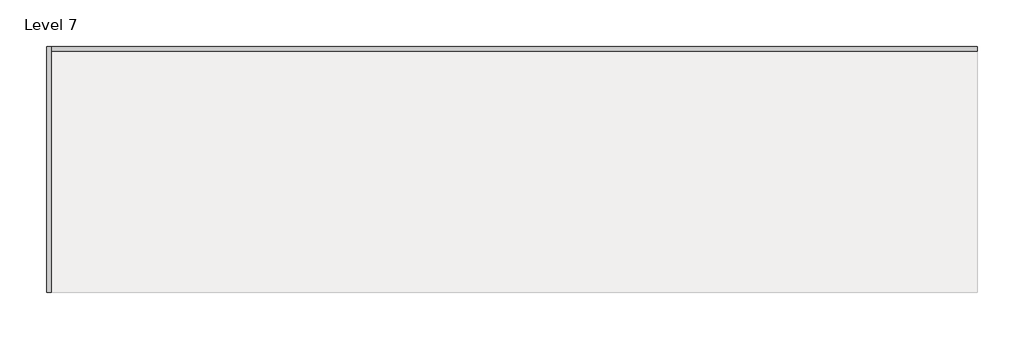
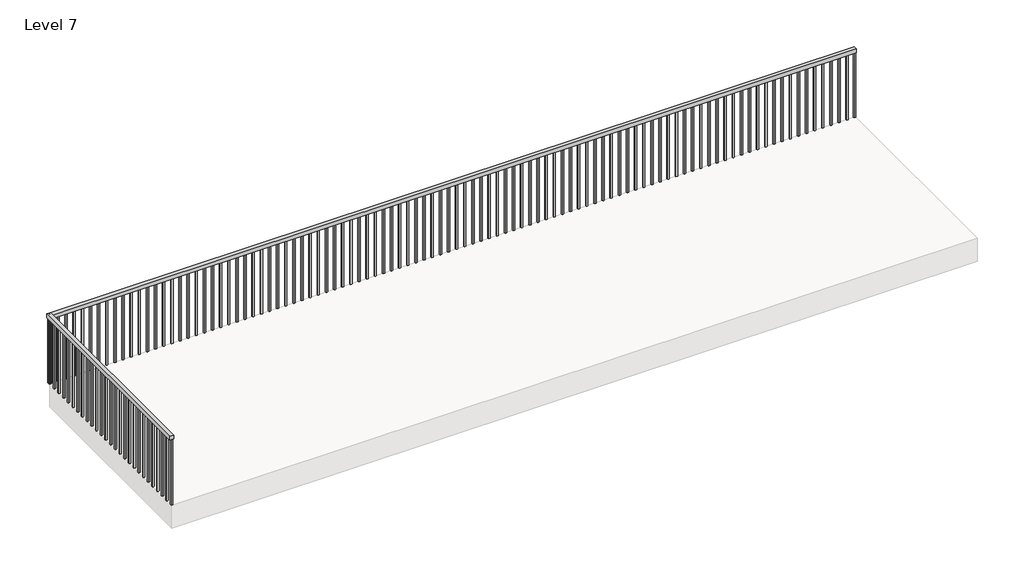
# One storey, part 3 of 5: 2 railings.
"""IFC4 building model written with IfcOpenShell, lengths in millimetres."""

from ifc_helpers import new_model, si_unit, frame, origin, place, context, project, spatial, polyline, outline, extrude, element, save

model = new_model("IFC4")

# Units and contexts
model_context = context("Model", 3, world=origin())
ifc_project = project(units=[si_unit("LENGTHUNIT", "METRE", prefix="MILLI")], contexts=[model_context])

# Site, building, storey
site = spatial("IfcSite", under=ifc_project)
building = spatial("IfcBuilding", under=site)
storey = spatial("IfcBuildingStorey", under=building, Name="Level 7", Elevation=6400.8)

# Railings
placement = place(None, origin())
element("IfcRailing", 1, ObjectType="Handrail - Rectangular", at=placement, inside=storey, context=model_context, shape_type="SweptSolid", body=[
    extrude(outline(polyline([(-13833.4638778, 17384.8237525), (-13833.4638778, 17435.6237525), (-3775.0638778, 17435.6237525), (-3775.0638778, 17384.8237525), (-13833.4638778, 17384.8237525)])), frame((0.0, 0.0, 7264.4), z_axis=(0.0, 0.0, 1.0), x_axis=(1.0, 0.0, 0.0)), (0.0, 0.0, 1.0), 50.8),
    extrude(outline(polyline([(-3886.1888778, 17400.6987525), (-3886.1888778, 17419.7487525), (-3867.1388778, 17419.7487525), (-3867.1388778, 17400.6987525), (-3886.1888778, 17400.6987525)])), frame((0.0, 0.0, 6400.8), z_axis=(0.0, 0.0, 1.0), x_axis=(1.0, 0.0, 0.0)), (0.0, 0.0, 1.0), 863.6),
    extrude(outline(polyline([(-3987.7888778, 17400.6987525), (-3987.7888778, 17419.7487525), (-3968.7388778, 17419.7487525), (-3968.7388778, 17400.6987525), (-3987.7888778, 17400.6987525)])), frame((0.0, 0.0, 6400.8), z_axis=(0.0, 0.0, 1.0), x_axis=(1.0, 0.0, 0.0)), (0.0, 0.0, 1.0), 863.6),
    extrude(outline(polyline([(-4089.3888778, 17400.6987525), (-4089.3888778, 17419.7487525), (-4070.3388778, 17419.7487525), (-4070.3388778, 17400.6987525), (-4089.3888778, 17400.6987525)])), frame((0.0, 0.0, 6400.8), z_axis=(0.0, 0.0, 1.0), x_axis=(1.0, 0.0, 0.0)), (0.0, 0.0, 1.0), 863.6),
    extrude(outline(polyline([(-4190.9888778, 17400.6987525), (-4190.9888778, 17419.7487525), (-4171.9388778, 17419.7487525), (-4171.9388778, 17400.6987525), (-4190.9888778, 17400.6987525)])), frame((0.0, 0.0, 6400.8), z_axis=(0.0, 0.0, 1.0), x_axis=(1.0, 0.0, 0.0)), (0.0, 0.0, 1.0), 863.6),
    extrude(outline(polyline([(-4292.5888778, 17400.6987525), (-4292.5888778, 17419.7487525), (-4273.5388778, 17419.7487525), (-4273.5388778, 17400.6987525), (-4292.5888778, 17400.6987525)])), frame((0.0, 0.0, 6400.8), z_axis=(0.0, 0.0, 1.0), x_axis=(1.0, 0.0, 0.0)), (0.0, 0.0, 1.0), 863.6),
    extrude(outline(polyline([(-4394.1888778, 17400.6987525), (-4394.1888778, 17419.7487525), (-4375.1388778, 17419.7487525), (-4375.1388778, 17400.6987525), (-4394.1888778, 17400.6987525)])), frame((0.0, 0.0, 6400.8), z_axis=(0.0, 0.0, 1.0), x_axis=(1.0, 0.0, 0.0)), (0.0, 0.0, 1.0), 863.6),
    extrude(outline(polyline([(-4495.7888778, 17400.6987525), (-4495.7888778, 17419.7487525), (-4476.7388778, 17419.7487525), (-4476.7388778, 17400.6987525), (-4495.7888778, 17400.6987525)])), frame((0.0, 0.0, 6400.8), z_axis=(0.0, 0.0, 1.0), x_axis=(1.0, 0.0, 0.0)), (0.0, 0.0, 1.0), 863.6),
    extrude(outline(polyline([(-4597.3888778, 17400.6987525), (-4597.3888778, 17419.7487525), (-4578.3388778, 17419.7487525), (-4578.3388778, 17400.6987525), (-4597.3888778, 17400.6987525)])), frame((0.0, 0.0, 6400.8), z_axis=(0.0, 0.0, 1.0), x_axis=(1.0, 0.0, 0.0)), (0.0, 0.0, 1.0), 863.6),
    extrude(outline(polyline([(-4698.9888778, 17400.6987525), (-4698.9888778, 17419.7487525), (-4679.9388778, 17419.7487525), (-4679.9388778, 17400.6987525), (-4698.9888778, 17400.6987525)])), frame((0.0, 0.0, 6400.8), z_axis=(0.0, 0.0, 1.0), x_axis=(1.0, 0.0, 0.0)), (0.0, 0.0, 1.0), 863.6),
    extrude(outline(polyline([(-4800.5888778, 17400.6987525), (-4800.5888778, 17419.7487525), (-4781.5388778, 17419.7487525), (-4781.5388778, 17400.6987525), (-4800.5888778, 17400.6987525)])), frame((0.0, 0.0, 6400.8), z_axis=(0.0, 0.0, 1.0), x_axis=(1.0, 0.0, 0.0)), (0.0, 0.0, 1.0), 863.6),
    extrude(outline(polyline([(-4902.1888778, 17400.6987525), (-4902.1888778, 17419.7487525), (-4883.1388778, 17419.7487525), (-4883.1388778, 17400.6987525), (-4902.1888778, 17400.6987525)])), frame((0.0, 0.0, 6400.8), z_axis=(0.0, 0.0, 1.0), x_axis=(1.0, 0.0, 0.0)), (0.0, 0.0, 1.0), 863.6),
    extrude(outline(polyline([(-5003.7888778, 17400.6987525), (-5003.7888778, 17419.7487525), (-4984.7388778, 17419.7487525), (-4984.7388778, 17400.6987525), (-5003.7888778, 17400.6987525)])), frame((0.0, 0.0, 6400.8), z_axis=(0.0, 0.0, 1.0), x_axis=(1.0, 0.0, 0.0)), (0.0, 0.0, 1.0), 863.6),
    extrude(outline(polyline([(-5105.3888778, 17400.6987525), (-5105.3888778, 17419.7487525), (-5086.3388778, 17419.7487525), (-5086.3388778, 17400.6987525), (-5105.3888778, 17400.6987525)])), frame((0.0, 0.0, 6400.8), z_axis=(0.0, 0.0, 1.0), x_axis=(1.0, 0.0, 0.0)), (0.0, 0.0, 1.0), 863.6),
    extrude(outline(polyline([(-5206.9888778, 17400.6987525), (-5206.9888778, 17419.7487525), (-5187.9388778, 17419.7487525), (-5187.9388778, 17400.6987525), (-5206.9888778, 17400.6987525)])), frame((0.0, 0.0, 6400.8), z_axis=(0.0, 0.0, 1.0), x_axis=(1.0, 0.0, 0.0)), (0.0, 0.0, 1.0), 863.6),
    extrude(outline(polyline([(-5308.5888778, 17400.6987525), (-5308.5888778, 17419.7487525), (-5289.5388778, 17419.7487525), (-5289.5388778, 17400.6987525), (-5308.5888778, 17400.6987525)])), frame((0.0, 0.0, 6400.8), z_axis=(0.0, 0.0, 1.0), x_axis=(1.0, 0.0, 0.0)), (0.0, 0.0, 1.0), 863.6),
    extrude(outline(polyline([(-5410.1888778, 17400.6987525), (-5410.1888778, 17419.7487525), (-5391.1388778, 17419.7487525), (-5391.1388778, 17400.6987525), (-5410.1888778, 17400.6987525)])), frame((0.0, 0.0, 6400.8), z_axis=(0.0, 0.0, 1.0), x_axis=(1.0, 0.0, 0.0)), (0.0, 0.0, 1.0), 863.6),
    extrude(outline(polyline([(-5511.7888778, 17400.6987525), (-5511.7888778, 17419.7487525), (-5492.7388778, 17419.7487525), (-5492.7388778, 17400.6987525), (-5511.7888778, 17400.6987525)])), frame((0.0, 0.0, 6400.8), z_axis=(0.0, 0.0, 1.0), x_axis=(1.0, 0.0, 0.0)), (0.0, 0.0, 1.0), 863.6),
    extrude(outline(polyline([(-5613.3888778, 17400.6987525), (-5613.3888778, 17419.7487525), (-5594.3388778, 17419.7487525), (-5594.3388778, 17400.6987525), (-5613.3888778, 17400.6987525)])), frame((0.0, 0.0, 6400.8), z_axis=(0.0, 0.0, 1.0), x_axis=(1.0, 0.0, 0.0)), (0.0, 0.0, 1.0), 863.6),
    extrude(outline(polyline([(-5714.9888778, 17400.6987525), (-5714.9888778, 17419.7487525), (-5695.9388778, 17419.7487525), (-5695.9388778, 17400.6987525), (-5714.9888778, 17400.6987525)])), frame((0.0, 0.0, 6400.8), z_axis=(0.0, 0.0, 1.0), x_axis=(1.0, 0.0, 0.0)), (0.0, 0.0, 1.0), 863.6),
    extrude(outline(polyline([(-5816.5888778, 17400.6987525), (-5816.5888778, 17419.7487525), (-5797.5388778, 17419.7487525), (-5797.5388778, 17400.6987525), (-5816.5888778, 17400.6987525)])), frame((0.0, 0.0, 6400.8), z_axis=(0.0, 0.0, 1.0), x_axis=(1.0, 0.0, 0.0)), (0.0, 0.0, 1.0), 863.6),
    extrude(outline(polyline([(-5918.1888778, 17400.6987525), (-5918.1888778, 17419.7487525), (-5899.1388778, 17419.7487525), (-5899.1388778, 17400.6987525), (-5918.1888778, 17400.6987525)])), frame((0.0, 0.0, 6400.8), z_axis=(0.0, 0.0, 1.0), x_axis=(1.0, 0.0, 0.0)), (0.0, 0.0, 1.0), 863.6),
    extrude(outline(polyline([(-6019.7888778, 17400.6987525), (-6019.7888778, 17419.7487525), (-6000.7388778, 17419.7487525), (-6000.7388778, 17400.6987525), (-6019.7888778, 17400.6987525)])), frame((0.0, 0.0, 6400.8), z_axis=(0.0, 0.0, 1.0), x_axis=(1.0, 0.0, 0.0)), (0.0, 0.0, 1.0), 863.6),
    extrude(outline(polyline([(-6121.3888778, 17400.6987525), (-6121.3888778, 17419.7487525), (-6102.3388778, 17419.7487525), (-6102.3388778, 17400.6987525), (-6121.3888778, 17400.6987525)])), frame((0.0, 0.0, 6400.8), z_axis=(0.0, 0.0, 1.0), x_axis=(1.0, 0.0, 0.0)), (0.0, 0.0, 1.0), 863.6),
    extrude(outline(polyline([(-6222.9888778, 17400.6987525), (-6222.9888778, 17419.7487525), (-6203.9388778, 17419.7487525), (-6203.9388778, 17400.6987525), (-6222.9888778, 17400.6987525)])), frame((0.0, 0.0, 6400.8), z_axis=(0.0, 0.0, 1.0), x_axis=(1.0, 0.0, 0.0)), (0.0, 0.0, 1.0), 863.6),
    extrude(outline(polyline([(-6324.5888778, 17400.6987525), (-6324.5888778, 17419.7487525), (-6305.5388778, 17419.7487525), (-6305.5388778, 17400.6987525), (-6324.5888778, 17400.6987525)])), frame((0.0, 0.0, 6400.8), z_axis=(0.0, 0.0, 1.0), x_axis=(1.0, 0.0, 0.0)), (0.0, 0.0, 1.0), 863.6),
    extrude(outline(polyline([(-6426.1888778, 17400.6987525), (-6426.1888778, 17419.7487525), (-6407.1388778, 17419.7487525), (-6407.1388778, 17400.6987525), (-6426.1888778, 17400.6987525)])), frame((0.0, 0.0, 6400.8), z_axis=(0.0, 0.0, 1.0), x_axis=(1.0, 0.0, 0.0)), (0.0, 0.0, 1.0), 863.6),
    extrude(outline(polyline([(-6527.7888778, 17400.6987525), (-6527.7888778, 17419.7487525), (-6508.7388778, 17419.7487525), (-6508.7388778, 17400.6987525), (-6527.7888778, 17400.6987525)])), frame((0.0, 0.0, 6400.8), z_axis=(0.0, 0.0, 1.0), x_axis=(1.0, 0.0, 0.0)), (0.0, 0.0, 1.0), 863.6),
    extrude(outline(polyline([(-6629.3888778, 17400.6987525), (-6629.3888778, 17419.7487525), (-6610.3388778, 17419.7487525), (-6610.3388778, 17400.6987525), (-6629.3888778, 17400.6987525)])), frame((0.0, 0.0, 6400.8), z_axis=(0.0, 0.0, 1.0), x_axis=(1.0, 0.0, 0.0)), (0.0, 0.0, 1.0), 863.6),
    extrude(outline(polyline([(-6730.9888778, 17400.6987525), (-6730.9888778, 17419.7487525), (-6711.9388778, 17419.7487525), (-6711.9388778, 17400.6987525), (-6730.9888778, 17400.6987525)])), frame((0.0, 0.0, 6400.8), z_axis=(0.0, 0.0, 1.0), x_axis=(1.0, 0.0, 0.0)), (0.0, 0.0, 1.0), 863.6),
    extrude(outline(polyline([(-6832.5888778, 17400.6987525), (-6832.5888778, 17419.7487525), (-6813.5388778, 17419.7487525), (-6813.5388778, 17400.6987525), (-6832.5888778, 17400.6987525)])), frame((0.0, 0.0, 6400.8), z_axis=(0.0, 0.0, 1.0), x_axis=(1.0, 0.0, 0.0)), (0.0, 0.0, 1.0), 863.6),
    extrude(outline(polyline([(-6934.1888778, 17400.6987525), (-6934.1888778, 17419.7487525), (-6915.1388778, 17419.7487525), (-6915.1388778, 17400.6987525), (-6934.1888778, 17400.6987525)])), frame((0.0, 0.0, 6400.8), z_axis=(0.0, 0.0, 1.0), x_axis=(1.0, 0.0, 0.0)), (0.0, 0.0, 1.0), 863.6),
    extrude(outline(polyline([(-7035.7888778, 17400.6987525), (-7035.7888778, 17419.7487525), (-7016.7388778, 17419.7487525), (-7016.7388778, 17400.6987525), (-7035.7888778, 17400.6987525)])), frame((0.0, 0.0, 6400.8), z_axis=(0.0, 0.0, 1.0), x_axis=(1.0, 0.0, 0.0)), (0.0, 0.0, 1.0), 863.6),
    extrude(outline(polyline([(-7137.3888778, 17400.6987525), (-7137.3888778, 17419.7487525), (-7118.3388778, 17419.7487525), (-7118.3388778, 17400.6987525), (-7137.3888778, 17400.6987525)])), frame((0.0, 0.0, 6400.8), z_axis=(0.0, 0.0, 1.0), x_axis=(1.0, 0.0, 0.0)), (0.0, 0.0, 1.0), 863.6),
    extrude(outline(polyline([(-7238.9888778, 17400.6987525), (-7238.9888778, 17419.7487525), (-7219.9388778, 17419.7487525), (-7219.9388778, 17400.6987525), (-7238.9888778, 17400.6987525)])), frame((0.0, 0.0, 6400.8), z_axis=(0.0, 0.0, 1.0), x_axis=(1.0, 0.0, 0.0)), (0.0, 0.0, 1.0), 863.6),
    extrude(outline(polyline([(-7340.5888778, 17400.6987525), (-7340.5888778, 17419.7487525), (-7321.5388778, 17419.7487525), (-7321.5388778, 17400.6987525), (-7340.5888778, 17400.6987525)])), frame((0.0, 0.0, 6400.8), z_axis=(0.0, 0.0, 1.0), x_axis=(1.0, 0.0, 0.0)), (0.0, 0.0, 1.0), 863.6),
    extrude(outline(polyline([(-7442.1888778, 17400.6987525), (-7442.1888778, 17419.7487525), (-7423.1388778, 17419.7487525), (-7423.1388778, 17400.6987525), (-7442.1888778, 17400.6987525)])), frame((0.0, 0.0, 6400.8), z_axis=(0.0, 0.0, 1.0), x_axis=(1.0, 0.0, 0.0)), (0.0, 0.0, 1.0), 863.6),
    extrude(outline(polyline([(-7543.7888778, 17400.6987525), (-7543.7888778, 17419.7487525), (-7524.7388778, 17419.7487525), (-7524.7388778, 17400.6987525), (-7543.7888778, 17400.6987525)])), frame((0.0, 0.0, 6400.8), z_axis=(0.0, 0.0, 1.0), x_axis=(1.0, 0.0, 0.0)), (0.0, 0.0, 1.0), 863.6),
    extrude(outline(polyline([(-7645.3888778, 17400.6987525), (-7645.3888778, 17419.7487525), (-7626.3388778, 17419.7487525), (-7626.3388778, 17400.6987525), (-7645.3888778, 17400.6987525)])), frame((0.0, 0.0, 6400.8), z_axis=(0.0, 0.0, 1.0), x_axis=(1.0, 0.0, 0.0)), (0.0, 0.0, 1.0), 863.6),
    extrude(outline(polyline([(-7746.9888778, 17400.6987525), (-7746.9888778, 17419.7487525), (-7727.9388778, 17419.7487525), (-7727.9388778, 17400.6987525), (-7746.9888778, 17400.6987525)])), frame((0.0, 0.0, 6400.8), z_axis=(0.0, 0.0, 1.0), x_axis=(1.0, 0.0, 0.0)), (0.0, 0.0, 1.0), 863.6),
    extrude(outline(polyline([(-7848.5888778, 17400.6987525), (-7848.5888778, 17419.7487525), (-7829.5388778, 17419.7487525), (-7829.5388778, 17400.6987525), (-7848.5888778, 17400.6987525)])), frame((0.0, 0.0, 6400.8), z_axis=(0.0, 0.0, 1.0), x_axis=(1.0, 0.0, 0.0)), (0.0, 0.0, 1.0), 863.6),
    extrude(outline(polyline([(-7950.1888778, 17400.6987525), (-7950.1888778, 17419.7487525), (-7931.1388778, 17419.7487525), (-7931.1388778, 17400.6987525), (-7950.1888778, 17400.6987525)])), frame((0.0, 0.0, 6400.8), z_axis=(0.0, 0.0, 1.0), x_axis=(1.0, 0.0, 0.0)), (0.0, 0.0, 1.0), 863.6),
    extrude(outline(polyline([(-8051.7888778, 17400.6987525), (-8051.7888778, 17419.7487525), (-8032.7388778, 17419.7487525), (-8032.7388778, 17400.6987525), (-8051.7888778, 17400.6987525)])), frame((0.0, 0.0, 6400.8), z_axis=(0.0, 0.0, 1.0), x_axis=(1.0, 0.0, 0.0)), (0.0, 0.0, 1.0), 863.6),
    extrude(outline(polyline([(-8153.3888778, 17400.6987525), (-8153.3888778, 17419.7487525), (-8134.3388778, 17419.7487525), (-8134.3388778, 17400.6987525), (-8153.3888778, 17400.6987525)])), frame((0.0, 0.0, 6400.8), z_axis=(0.0, 0.0, 1.0), x_axis=(1.0, 0.0, 0.0)), (0.0, 0.0, 1.0), 863.6),
    extrude(outline(polyline([(-8254.9888778, 17400.6987525), (-8254.9888778, 17419.7487525), (-8235.9388778, 17419.7487525), (-8235.9388778, 17400.6987525), (-8254.9888778, 17400.6987525)])), frame((0.0, 0.0, 6400.8), z_axis=(0.0, 0.0, 1.0), x_axis=(1.0, 0.0, 0.0)), (0.0, 0.0, 1.0), 863.6),
    extrude(outline(polyline([(-8356.5888778, 17400.6987525), (-8356.5888778, 17419.7487525), (-8337.5388778, 17419.7487525), (-8337.5388778, 17400.6987525), (-8356.5888778, 17400.6987525)])), frame((0.0, 0.0, 6400.8), z_axis=(0.0, 0.0, 1.0), x_axis=(1.0, 0.0, 0.0)), (0.0, 0.0, 1.0), 863.6),
    extrude(outline(polyline([(-8458.1888778, 17400.6987525), (-8458.1888778, 17419.7487525), (-8439.1388778, 17419.7487525), (-8439.1388778, 17400.6987525), (-8458.1888778, 17400.6987525)])), frame((0.0, 0.0, 6400.8), z_axis=(0.0, 0.0, 1.0), x_axis=(1.0, 0.0, 0.0)), (0.0, 0.0, 1.0), 863.6),
    extrude(outline(polyline([(-8559.7888778, 17400.6987525), (-8559.7888778, 17419.7487525), (-8540.7388778, 17419.7487525), (-8540.7388778, 17400.6987525), (-8559.7888778, 17400.6987525)])), frame((0.0, 0.0, 6400.8), z_axis=(0.0, 0.0, 1.0), x_axis=(1.0, 0.0, 0.0)), (0.0, 0.0, 1.0), 863.6),
    extrude(outline(polyline([(-8661.3888778, 17400.6987525), (-8661.3888778, 17419.7487525), (-8642.3388778, 17419.7487525), (-8642.3388778, 17400.6987525), (-8661.3888778, 17400.6987525)])), frame((0.0, 0.0, 6400.8), z_axis=(0.0, 0.0, 1.0), x_axis=(1.0, 0.0, 0.0)), (0.0, 0.0, 1.0), 863.6),
    extrude(outline(polyline([(-8762.9888778, 17400.6987525), (-8762.9888778, 17419.7487525), (-8743.9388778, 17419.7487525), (-8743.9388778, 17400.6987525), (-8762.9888778, 17400.6987525)])), frame((0.0, 0.0, 6400.8), z_axis=(0.0, 0.0, 1.0), x_axis=(1.0, 0.0, 0.0)), (0.0, 0.0, 1.0), 863.6),
    extrude(outline(polyline([(-8864.5888778, 17400.6987525), (-8864.5888778, 17419.7487525), (-8845.5388778, 17419.7487525), (-8845.5388778, 17400.6987525), (-8864.5888778, 17400.6987525)])), frame((0.0, 0.0, 6400.8), z_axis=(0.0, 0.0, 1.0), x_axis=(1.0, 0.0, 0.0)), (0.0, 0.0, 1.0), 863.6),
    extrude(outline(polyline([(-8966.1888778, 17400.6987525), (-8966.1888778, 17419.7487525), (-8947.1388778, 17419.7487525), (-8947.1388778, 17400.6987525), (-8966.1888778, 17400.6987525)])), frame((0.0, 0.0, 6400.8), z_axis=(0.0, 0.0, 1.0), x_axis=(1.0, 0.0, 0.0)), (0.0, 0.0, 1.0), 863.6),
    extrude(outline(polyline([(-9067.7888778, 17400.6987525), (-9067.7888778, 17419.7487525), (-9048.7388778, 17419.7487525), (-9048.7388778, 17400.6987525), (-9067.7888778, 17400.6987525)])), frame((0.0, 0.0, 6400.8), z_axis=(0.0, 0.0, 1.0), x_axis=(1.0, 0.0, 0.0)), (0.0, 0.0, 1.0), 863.6),
    extrude(outline(polyline([(-9169.3888778, 17400.6987525), (-9169.3888778, 17419.7487525), (-9150.3388778, 17419.7487525), (-9150.3388778, 17400.6987525), (-9169.3888778, 17400.6987525)])), frame((0.0, 0.0, 6400.8), z_axis=(0.0, 0.0, 1.0), x_axis=(1.0, 0.0, 0.0)), (0.0, 0.0, 1.0), 863.6),
    extrude(outline(polyline([(-9270.9888778, 17400.6987525), (-9270.9888778, 17419.7487525), (-9251.9388778, 17419.7487525), (-9251.9388778, 17400.6987525), (-9270.9888778, 17400.6987525)])), frame((0.0, 0.0, 6400.8), z_axis=(0.0, 0.0, 1.0), x_axis=(1.0, 0.0, 0.0)), (0.0, 0.0, 1.0), 863.6),
    extrude(outline(polyline([(-9372.5888778, 17400.6987525), (-9372.5888778, 17419.7487525), (-9353.5388778, 17419.7487525), (-9353.5388778, 17400.6987525), (-9372.5888778, 17400.6987525)])), frame((0.0, 0.0, 6400.8), z_axis=(0.0, 0.0, 1.0), x_axis=(1.0, 0.0, 0.0)), (0.0, 0.0, 1.0), 863.6),
    extrude(outline(polyline([(-9474.1888778, 17400.6987525), (-9474.1888778, 17419.7487525), (-9455.1388778, 17419.7487525), (-9455.1388778, 17400.6987525), (-9474.1888778, 17400.6987525)])), frame((0.0, 0.0, 6400.8), z_axis=(0.0, 0.0, 1.0), x_axis=(1.0, 0.0, 0.0)), (0.0, 0.0, 1.0), 863.6),
    extrude(outline(polyline([(-9575.7888778, 17400.6987525), (-9575.7888778, 17419.7487525), (-9556.7388778, 17419.7487525), (-9556.7388778, 17400.6987525), (-9575.7888778, 17400.6987525)])), frame((0.0, 0.0, 6400.8), z_axis=(0.0, 0.0, 1.0), x_axis=(1.0, 0.0, 0.0)), (0.0, 0.0, 1.0), 863.6),
    extrude(outline(polyline([(-9677.3888778, 17400.6987525), (-9677.3888778, 17419.7487525), (-9658.3388778, 17419.7487525), (-9658.3388778, 17400.6987525), (-9677.3888778, 17400.6987525)])), frame((0.0, 0.0, 6400.8), z_axis=(0.0, 0.0, 1.0), x_axis=(1.0, 0.0, 0.0)), (0.0, 0.0, 1.0), 863.6),
    extrude(outline(polyline([(-9778.9888778, 17400.6987525), (-9778.9888778, 17419.7487525), (-9759.9388778, 17419.7487525), (-9759.9388778, 17400.6987525), (-9778.9888778, 17400.6987525)])), frame((0.0, 0.0, 6400.8), z_axis=(0.0, 0.0, 1.0), x_axis=(1.0, 0.0, 0.0)), (0.0, 0.0, 1.0), 863.6),
    extrude(outline(polyline([(-9880.5888778, 17400.6987525), (-9880.5888778, 17419.7487525), (-9861.5388778, 17419.7487525), (-9861.5388778, 17400.6987525), (-9880.5888778, 17400.6987525)])), frame((0.0, 0.0, 6400.8), z_axis=(0.0, 0.0, 1.0), x_axis=(1.0, 0.0, 0.0)), (0.0, 0.0, 1.0), 863.6),
    extrude(outline(polyline([(-9982.1888778, 17400.6987525), (-9982.1888778, 17419.7487525), (-9963.1388778, 17419.7487525), (-9963.1388778, 17400.6987525), (-9982.1888778, 17400.6987525)])), frame((0.0, 0.0, 6400.8), z_axis=(0.0, 0.0, 1.0), x_axis=(1.0, 0.0, 0.0)), (0.0, 0.0, 1.0), 863.6),
    extrude(outline(polyline([(-10083.7888778, 17400.6987525), (-10083.7888778, 17419.7487525), (-10064.7388778, 17419.7487525), (-10064.7388778, 17400.6987525), (-10083.7888778, 17400.6987525)])), frame((0.0, 0.0, 6400.8), z_axis=(0.0, 0.0, 1.0), x_axis=(1.0, 0.0, 0.0)), (0.0, 0.0, 1.0), 863.6),
    extrude(outline(polyline([(-10185.3888778, 17400.6987525), (-10185.3888778, 17419.7487525), (-10166.3388778, 17419.7487525), (-10166.3388778, 17400.6987525), (-10185.3888778, 17400.6987525)])), frame((0.0, 0.0, 6400.8), z_axis=(0.0, 0.0, 1.0), x_axis=(1.0, 0.0, 0.0)), (0.0, 0.0, 1.0), 863.6),
    extrude(outline(polyline([(-10286.9888778, 17400.6987525), (-10286.9888778, 17419.7487525), (-10267.9388778, 17419.7487525), (-10267.9388778, 17400.6987525), (-10286.9888778, 17400.6987525)])), frame((0.0, 0.0, 6400.8), z_axis=(0.0, 0.0, 1.0), x_axis=(1.0, 0.0, 0.0)), (0.0, 0.0, 1.0), 863.6),
    extrude(outline(polyline([(-10388.5888778, 17400.6987525), (-10388.5888778, 17419.7487525), (-10369.5388778, 17419.7487525), (-10369.5388778, 17400.6987525), (-10388.5888778, 17400.6987525)])), frame((0.0, 0.0, 6400.8), z_axis=(0.0, 0.0, 1.0), x_axis=(1.0, 0.0, 0.0)), (0.0, 0.0, 1.0), 863.6),
    extrude(outline(polyline([(-10490.1888778, 17400.6987525), (-10490.1888778, 17419.7487525), (-10471.1388778, 17419.7487525), (-10471.1388778, 17400.6987525), (-10490.1888778, 17400.6987525)])), frame((0.0, 0.0, 6400.8), z_axis=(0.0, 0.0, 1.0), x_axis=(1.0, 0.0, 0.0)), (0.0, 0.0, 1.0), 863.6),
    extrude(outline(polyline([(-10591.7888778, 17400.6987525), (-10591.7888778, 17419.7487525), (-10572.7388778, 17419.7487525), (-10572.7388778, 17400.6987525), (-10591.7888778, 17400.6987525)])), frame((0.0, 0.0, 6400.8), z_axis=(0.0, 0.0, 1.0), x_axis=(1.0, 0.0, 0.0)), (0.0, 0.0, 1.0), 863.6),
    extrude(outline(polyline([(-10693.3888778, 17400.6987525), (-10693.3888778, 17419.7487525), (-10674.3388778, 17419.7487525), (-10674.3388778, 17400.6987525), (-10693.3888778, 17400.6987525)])), frame((0.0, 0.0, 6400.8), z_axis=(0.0, 0.0, 1.0), x_axis=(1.0, 0.0, 0.0)), (0.0, 0.0, 1.0), 863.6),
    extrude(outline(polyline([(-10794.9888778, 17400.6987525), (-10794.9888778, 17419.7487525), (-10775.9388778, 17419.7487525), (-10775.9388778, 17400.6987525), (-10794.9888778, 17400.6987525)])), frame((0.0, 0.0, 6400.8), z_axis=(0.0, 0.0, 1.0), x_axis=(1.0, 0.0, 0.0)), (0.0, 0.0, 1.0), 863.6),
    extrude(outline(polyline([(-10896.5888778, 17400.6987525), (-10896.5888778, 17419.7487525), (-10877.5388778, 17419.7487525), (-10877.5388778, 17400.6987525), (-10896.5888778, 17400.6987525)])), frame((0.0, 0.0, 6400.8), z_axis=(0.0, 0.0, 1.0), x_axis=(1.0, 0.0, 0.0)), (0.0, 0.0, 1.0), 863.6),
    extrude(outline(polyline([(-10998.1888778, 17400.6987525), (-10998.1888778, 17419.7487525), (-10979.1388778, 17419.7487525), (-10979.1388778, 17400.6987525), (-10998.1888778, 17400.6987525)])), frame((0.0, 0.0, 6400.8), z_axis=(0.0, 0.0, 1.0), x_axis=(1.0, 0.0, 0.0)), (0.0, 0.0, 1.0), 863.6),
    extrude(outline(polyline([(-11099.7888778, 17400.6987525), (-11099.7888778, 17419.7487525), (-11080.7388778, 17419.7487525), (-11080.7388778, 17400.6987525), (-11099.7888778, 17400.6987525)])), frame((0.0, 0.0, 6400.8), z_axis=(0.0, 0.0, 1.0), x_axis=(1.0, 0.0, 0.0)), (0.0, 0.0, 1.0), 863.6),
    extrude(outline(polyline([(-11201.3888778, 17400.6987525), (-11201.3888778, 17419.7487525), (-11182.3388778, 17419.7487525), (-11182.3388778, 17400.6987525), (-11201.3888778, 17400.6987525)])), frame((0.0, 0.0, 6400.8), z_axis=(0.0, 0.0, 1.0), x_axis=(1.0, 0.0, 0.0)), (0.0, 0.0, 1.0), 863.6),
    extrude(outline(polyline([(-11302.9888778, 17400.6987525), (-11302.9888778, 17419.7487525), (-11283.9388778, 17419.7487525), (-11283.9388778, 17400.6987525), (-11302.9888778, 17400.6987525)])), frame((0.0, 0.0, 6400.8), z_axis=(0.0, 0.0, 1.0), x_axis=(1.0, 0.0, 0.0)), (0.0, 0.0, 1.0), 863.6),
    extrude(outline(polyline([(-11404.5888778, 17400.6987525), (-11404.5888778, 17419.7487525), (-11385.5388778, 17419.7487525), (-11385.5388778, 17400.6987525), (-11404.5888778, 17400.6987525)])), frame((0.0, 0.0, 6400.8), z_axis=(0.0, 0.0, 1.0), x_axis=(1.0, 0.0, 0.0)), (0.0, 0.0, 1.0), 863.6),
    extrude(outline(polyline([(-11506.1888778, 17400.6987525), (-11506.1888778, 17419.7487525), (-11487.1388778, 17419.7487525), (-11487.1388778, 17400.6987525), (-11506.1888778, 17400.6987525)])), frame((0.0, 0.0, 6400.8), z_axis=(0.0, 0.0, 1.0), x_axis=(1.0, 0.0, 0.0)), (0.0, 0.0, 1.0), 863.6),
    extrude(outline(polyline([(-11607.7888778, 17400.6987525), (-11607.7888778, 17419.7487525), (-11588.7388778, 17419.7487525), (-11588.7388778, 17400.6987525), (-11607.7888778, 17400.6987525)])), frame((0.0, 0.0, 6400.8), z_axis=(0.0, 0.0, 1.0), x_axis=(1.0, 0.0, 0.0)), (0.0, 0.0, 1.0), 863.6),
    extrude(outline(polyline([(-11709.3888778, 17400.6987525), (-11709.3888778, 17419.7487525), (-11690.3388778, 17419.7487525), (-11690.3388778, 17400.6987525), (-11709.3888778, 17400.6987525)])), frame((0.0, 0.0, 6400.8), z_axis=(0.0, 0.0, 1.0), x_axis=(1.0, 0.0, 0.0)), (0.0, 0.0, 1.0), 863.6),
    extrude(outline(polyline([(-11810.9888778, 17400.6987525), (-11810.9888778, 17419.7487525), (-11791.9388778, 17419.7487525), (-11791.9388778, 17400.6987525), (-11810.9888778, 17400.6987525)])), frame((0.0, 0.0, 6400.8), z_axis=(0.0, 0.0, 1.0), x_axis=(1.0, 0.0, 0.0)), (0.0, 0.0, 1.0), 863.6),
    extrude(outline(polyline([(-11912.5888778, 17400.6987525), (-11912.5888778, 17419.7487525), (-11893.5388778, 17419.7487525), (-11893.5388778, 17400.6987525), (-11912.5888778, 17400.6987525)])), frame((0.0, 0.0, 6400.8), z_axis=(0.0, 0.0, 1.0), x_axis=(1.0, 0.0, 0.0)), (0.0, 0.0, 1.0), 863.6),
    extrude(outline(polyline([(-12014.1888778, 17400.6987525), (-12014.1888778, 17419.7487525), (-11995.1388778, 17419.7487525), (-11995.1388778, 17400.6987525), (-12014.1888778, 17400.6987525)])), frame((0.0, 0.0, 6400.8), z_axis=(0.0, 0.0, 1.0), x_axis=(1.0, 0.0, 0.0)), (0.0, 0.0, 1.0), 863.6),
    extrude(outline(polyline([(-12115.7888778, 17400.6987525), (-12115.7888778, 17419.7487525), (-12096.7388778, 17419.7487525), (-12096.7388778, 17400.6987525), (-12115.7888778, 17400.6987525)])), frame((0.0, 0.0, 6400.8), z_axis=(0.0, 0.0, 1.0), x_axis=(1.0, 0.0, 0.0)), (0.0, 0.0, 1.0), 863.6),
    extrude(outline(polyline([(-12217.3888778, 17400.6987525), (-12217.3888778, 17419.7487525), (-12198.3388778, 17419.7487525), (-12198.3388778, 17400.6987525), (-12217.3888778, 17400.6987525)])), frame((0.0, 0.0, 6400.8), z_axis=(0.0, 0.0, 1.0), x_axis=(1.0, 0.0, 0.0)), (0.0, 0.0, 1.0), 863.6),
    extrude(outline(polyline([(-12318.9888778, 17400.6987525), (-12318.9888778, 17419.7487525), (-12299.9388778, 17419.7487525), (-12299.9388778, 17400.6987525), (-12318.9888778, 17400.6987525)])), frame((0.0, 0.0, 6400.8), z_axis=(0.0, 0.0, 1.0), x_axis=(1.0, 0.0, 0.0)), (0.0, 0.0, 1.0), 863.6),
    extrude(outline(polyline([(-12420.5888778, 17400.6987525), (-12420.5888778, 17419.7487525), (-12401.5388778, 17419.7487525), (-12401.5388778, 17400.6987525), (-12420.5888778, 17400.6987525)])), frame((0.0, 0.0, 6400.8), z_axis=(0.0, 0.0, 1.0), x_axis=(1.0, 0.0, 0.0)), (0.0, 0.0, 1.0), 863.6),
    extrude(outline(polyline([(-12522.1888778, 17400.6987525), (-12522.1888778, 17419.7487525), (-12503.1388778, 17419.7487525), (-12503.1388778, 17400.6987525), (-12522.1888778, 17400.6987525)])), frame((0.0, 0.0, 6400.8), z_axis=(0.0, 0.0, 1.0), x_axis=(1.0, 0.0, 0.0)), (0.0, 0.0, 1.0), 863.6),
    extrude(outline(polyline([(-12623.7888778, 17400.6987525), (-12623.7888778, 17419.7487525), (-12604.7388778, 17419.7487525), (-12604.7388778, 17400.6987525), (-12623.7888778, 17400.6987525)])), frame((0.0, 0.0, 6400.8), z_axis=(0.0, 0.0, 1.0), x_axis=(1.0, 0.0, 0.0)), (0.0, 0.0, 1.0), 863.6),
    extrude(outline(polyline([(-12725.3888778, 17400.6987525), (-12725.3888778, 17419.7487525), (-12706.3388778, 17419.7487525), (-12706.3388778, 17400.6987525), (-12725.3888778, 17400.6987525)])), frame((0.0, 0.0, 6400.8), z_axis=(0.0, 0.0, 1.0), x_axis=(1.0, 0.0, 0.0)), (0.0, 0.0, 1.0), 863.6),
    extrude(outline(polyline([(-12826.9888778, 17400.6987525), (-12826.9888778, 17419.7487525), (-12807.9388778, 17419.7487525), (-12807.9388778, 17400.6987525), (-12826.9888778, 17400.6987525)])), frame((0.0, 0.0, 6400.8), z_axis=(0.0, 0.0, 1.0), x_axis=(1.0, 0.0, 0.0)), (0.0, 0.0, 1.0), 863.6),
    extrude(outline(polyline([(-12928.5888778, 17400.6987525), (-12928.5888778, 17419.7487525), (-12909.5388778, 17419.7487525), (-12909.5388778, 17400.6987525), (-12928.5888778, 17400.6987525)])), frame((0.0, 0.0, 6400.8), z_axis=(0.0, 0.0, 1.0), x_axis=(1.0, 0.0, 0.0)), (0.0, 0.0, 1.0), 863.6),
    extrude(outline(polyline([(-13030.1888778, 17400.6987525), (-13030.1888778, 17419.7487525), (-13011.1388778, 17419.7487525), (-13011.1388778, 17400.6987525), (-13030.1888778, 17400.6987525)])), frame((0.0, 0.0, 6400.8), z_axis=(0.0, 0.0, 1.0), x_axis=(1.0, 0.0, 0.0)), (0.0, 0.0, 1.0), 863.6),
    extrude(outline(polyline([(-13131.7888778, 17400.6987525), (-13131.7888778, 17419.7487525), (-13112.7388778, 17419.7487525), (-13112.7388778, 17400.6987525), (-13131.7888778, 17400.6987525)])), frame((0.0, 0.0, 6400.8), z_axis=(0.0, 0.0, 1.0), x_axis=(1.0, 0.0, 0.0)), (0.0, 0.0, 1.0), 863.6),
    extrude(outline(polyline([(-13233.3888778, 17400.6987525), (-13233.3888778, 17419.7487525), (-13214.3388778, 17419.7487525), (-13214.3388778, 17400.6987525), (-13233.3888778, 17400.6987525)])), frame((0.0, 0.0, 6400.8), z_axis=(0.0, 0.0, 1.0), x_axis=(1.0, 0.0, 0.0)), (0.0, 0.0, 1.0), 863.6),
    extrude(outline(polyline([(-13334.9888778, 17400.6987525), (-13334.9888778, 17419.7487525), (-13315.9388778, 17419.7487525), (-13315.9388778, 17400.6987525), (-13334.9888778, 17400.6987525)])), frame((0.0, 0.0, 6400.8), z_axis=(0.0, 0.0, 1.0), x_axis=(1.0, 0.0, 0.0)), (0.0, 0.0, 1.0), 863.6),
    extrude(outline(polyline([(-13436.5888778, 17400.6987525), (-13436.5888778, 17419.7487525), (-13417.5388778, 17419.7487525), (-13417.5388778, 17400.6987525), (-13436.5888778, 17400.6987525)])), frame((0.0, 0.0, 6400.8), z_axis=(0.0, 0.0, 1.0), x_axis=(1.0, 0.0, 0.0)), (0.0, 0.0, 1.0), 863.6),
    extrude(outline(polyline([(-13538.1888778, 17400.6987525), (-13538.1888778, 17419.7487525), (-13519.1388778, 17419.7487525), (-13519.1388778, 17400.6987525), (-13538.1888778, 17400.6987525)])), frame((0.0, 0.0, 6400.8), z_axis=(0.0, 0.0, 1.0), x_axis=(1.0, 0.0, 0.0)), (0.0, 0.0, 1.0), 863.6),
    extrude(outline(polyline([(-13639.7888778, 17400.6987525), (-13639.7888778, 17419.7487525), (-13620.7388778, 17419.7487525), (-13620.7388778, 17400.6987525), (-13639.7888778, 17400.6987525)])), frame((0.0, 0.0, 6400.8), z_axis=(0.0, 0.0, 1.0), x_axis=(1.0, 0.0, 0.0)), (0.0, 0.0, 1.0), 863.6),
    extrude(outline(polyline([(-13741.3888778, 17400.6987525), (-13741.3888778, 17419.7487525), (-13722.3388778, 17419.7487525), (-13722.3388778, 17400.6987525), (-13741.3888778, 17400.6987525)])), frame((0.0, 0.0, 6400.8), z_axis=(0.0, 0.0, 1.0), x_axis=(1.0, 0.0, 0.0)), (0.0, 0.0, 1.0), 863.6),
    extrude(outline(polyline([(-3794.1138778, 17400.6987525), (-3794.1138778, 17419.7487525), (-3775.0638778, 17419.7487525), (-3775.0638778, 17400.6987525), (-3794.1138778, 17400.6987525)])), frame((0.0, 0.0, 6400.8), z_axis=(0.0, 0.0, 1.0), x_axis=(1.0, 0.0, 0.0)), (0.0, 0.0, 1.0), 863.6),
    extrude(outline(polyline([(-13833.4638778, 17400.6987525), (-13833.4638778, 17419.7487525), (-13814.4138778, 17419.7487525), (-13814.4138778, 17400.6987525), (-13833.4638778, 17400.6987525)])), frame((0.0, 0.0, 6400.8), z_axis=(0.0, 0.0, 1.0), x_axis=(1.0, 0.0, 0.0)), (0.0, 0.0, 1.0), 863.6),
])
element("IfcRailing", 2, ObjectType="Handrail - Rectangular", at=placement, inside=storey, context=model_context, shape_type="SweptSolid", body=[
    extrude(outline(polyline([(-13808.0638778, 14768.6237525), (-13858.8638778, 14768.6237525), (-13858.8638778, 17435.6237525), (-13808.0638778, 17435.6237525), (-13808.0638778, 14768.6237525)])), frame((0.0, 0.0, 7264.4), z_axis=(0.0, 0.0, 1.0), x_axis=(1.0, 0.0, 0.0)), (0.0, 0.0, 1.0), 50.8),
    extrude(outline(polyline([(-13823.9388778, 17400.6987525), (-13842.9888778, 17400.6987525), (-13842.9888778, 17419.7487525), (-13823.9388778, 17419.7487525), (-13823.9388778, 17400.6987525)])), frame((0.0, 0.0, 6400.8), z_axis=(0.0, 0.0, 1.0), x_axis=(1.0, 0.0, 0.0)), (0.0, 0.0, 1.0), 863.6),
    extrude(outline(polyline([(-13823.9388778, 17299.0987525), (-13842.9888778, 17299.0987525), (-13842.9888778, 17318.1487525), (-13823.9388778, 17318.1487525), (-13823.9388778, 17299.0987525)])), frame((0.0, 0.0, 6400.8), z_axis=(0.0, 0.0, 1.0), x_axis=(1.0, 0.0, 0.0)), (0.0, 0.0, 1.0), 863.6),
    extrude(outline(polyline([(-13823.9388778, 17197.4987525), (-13842.9888778, 17197.4987525), (-13842.9888778, 17216.5487525), (-13823.9388778, 17216.5487525), (-13823.9388778, 17197.4987525)])), frame((0.0, 0.0, 6400.8), z_axis=(0.0, 0.0, 1.0), x_axis=(1.0, 0.0, 0.0)), (0.0, 0.0, 1.0), 863.6),
    extrude(outline(polyline([(-13823.9388778, 17095.8987525), (-13842.9888778, 17095.8987525), (-13842.9888778, 17114.9487525), (-13823.9388778, 17114.9487525), (-13823.9388778, 17095.8987525)])), frame((0.0, 0.0, 6400.8), z_axis=(0.0, 0.0, 1.0), x_axis=(1.0, 0.0, 0.0)), (0.0, 0.0, 1.0), 863.6),
    extrude(outline(polyline([(-13823.9388778, 16994.2987525), (-13842.9888778, 16994.2987525), (-13842.9888778, 17013.3487525), (-13823.9388778, 17013.3487525), (-13823.9388778, 16994.2987525)])), frame((0.0, 0.0, 6400.8), z_axis=(0.0, 0.0, 1.0), x_axis=(1.0, 0.0, 0.0)), (0.0, 0.0, 1.0), 863.6),
    extrude(outline(polyline([(-13823.9388778, 16892.6987525), (-13842.9888778, 16892.6987525), (-13842.9888778, 16911.7487525), (-13823.9388778, 16911.7487525), (-13823.9388778, 16892.6987525)])), frame((0.0, 0.0, 6400.8), z_axis=(0.0, 0.0, 1.0), x_axis=(1.0, 0.0, 0.0)), (0.0, 0.0, 1.0), 863.6),
    extrude(outline(polyline([(-13823.9388778, 16791.0987525), (-13842.9888778, 16791.0987525), (-13842.9888778, 16810.1487525), (-13823.9388778, 16810.1487525), (-13823.9388778, 16791.0987525)])), frame((0.0, 0.0, 6400.8), z_axis=(0.0, 0.0, 1.0), x_axis=(1.0, 0.0, 0.0)), (0.0, 0.0, 1.0), 863.6),
    extrude(outline(polyline([(-13823.9388778, 16689.4987525), (-13842.9888778, 16689.4987525), (-13842.9888778, 16708.5487525), (-13823.9388778, 16708.5487525), (-13823.9388778, 16689.4987525)])), frame((0.0, 0.0, 6400.8), z_axis=(0.0, 0.0, 1.0), x_axis=(1.0, 0.0, 0.0)), (0.0, 0.0, 1.0), 863.6),
    extrude(outline(polyline([(-13823.9388778, 16587.8987525), (-13842.9888778, 16587.8987525), (-13842.9888778, 16606.9487525), (-13823.9388778, 16606.9487525), (-13823.9388778, 16587.8987525)])), frame((0.0, 0.0, 6400.8), z_axis=(0.0, 0.0, 1.0), x_axis=(1.0, 0.0, 0.0)), (0.0, 0.0, 1.0), 863.6),
    extrude(outline(polyline([(-13823.9388778, 16486.2987525), (-13842.9888778, 16486.2987525), (-13842.9888778, 16505.3487525), (-13823.9388778, 16505.3487525), (-13823.9388778, 16486.2987525)])), frame((0.0, 0.0, 6400.8), z_axis=(0.0, 0.0, 1.0), x_axis=(1.0, 0.0, 0.0)), (0.0, 0.0, 1.0), 863.6),
    extrude(outline(polyline([(-13823.9388778, 16384.6987525), (-13842.9888778, 16384.6987525), (-13842.9888778, 16403.7487525), (-13823.9388778, 16403.7487525), (-13823.9388778, 16384.6987525)])), frame((0.0, 0.0, 6400.8), z_axis=(0.0, 0.0, 1.0), x_axis=(1.0, 0.0, 0.0)), (0.0, 0.0, 1.0), 863.6),
    extrude(outline(polyline([(-13823.9388778, 16283.0987525), (-13842.9888778, 16283.0987525), (-13842.9888778, 16302.1487525), (-13823.9388778, 16302.1487525), (-13823.9388778, 16283.0987525)])), frame((0.0, 0.0, 6400.8), z_axis=(0.0, 0.0, 1.0), x_axis=(1.0, 0.0, 0.0)), (0.0, 0.0, 1.0), 863.6),
    extrude(outline(polyline([(-13823.9388778, 16181.4987525), (-13842.9888778, 16181.4987525), (-13842.9888778, 16200.5487525), (-13823.9388778, 16200.5487525), (-13823.9388778, 16181.4987525)])), frame((0.0, 0.0, 6400.8), z_axis=(0.0, 0.0, 1.0), x_axis=(1.0, 0.0, 0.0)), (0.0, 0.0, 1.0), 863.6),
    extrude(outline(polyline([(-13823.9388778, 16079.8987525), (-13842.9888778, 16079.8987525), (-13842.9888778, 16098.9487525), (-13823.9388778, 16098.9487525), (-13823.9388778, 16079.8987525)])), frame((0.0, 0.0, 6400.8), z_axis=(0.0, 0.0, 1.0), x_axis=(1.0, 0.0, 0.0)), (0.0, 0.0, 1.0), 863.6),
    extrude(outline(polyline([(-13823.9388778, 15978.2987525), (-13842.9888778, 15978.2987525), (-13842.9888778, 15997.3487525), (-13823.9388778, 15997.3487525), (-13823.9388778, 15978.2987525)])), frame((0.0, 0.0, 6400.8), z_axis=(0.0, 0.0, 1.0), x_axis=(1.0, 0.0, 0.0)), (0.0, 0.0, 1.0), 863.6),
    extrude(outline(polyline([(-13823.9388778, 15876.6987525), (-13842.9888778, 15876.6987525), (-13842.9888778, 15895.7487525), (-13823.9388778, 15895.7487525), (-13823.9388778, 15876.6987525)])), frame((0.0, 0.0, 6400.8), z_axis=(0.0, 0.0, 1.0), x_axis=(1.0, 0.0, 0.0)), (0.0, 0.0, 1.0), 863.6),
    extrude(outline(polyline([(-13823.9388778, 15775.0987525), (-13842.9888778, 15775.0987525), (-13842.9888778, 15794.1487525), (-13823.9388778, 15794.1487525), (-13823.9388778, 15775.0987525)])), frame((0.0, 0.0, 6400.8), z_axis=(0.0, 0.0, 1.0), x_axis=(1.0, 0.0, 0.0)), (0.0, 0.0, 1.0), 863.6),
    extrude(outline(polyline([(-13823.9388778, 15673.4987525), (-13842.9888778, 15673.4987525), (-13842.9888778, 15692.5487525), (-13823.9388778, 15692.5487525), (-13823.9388778, 15673.4987525)])), frame((0.0, 0.0, 6400.8), z_axis=(0.0, 0.0, 1.0), x_axis=(1.0, 0.0, 0.0)), (0.0, 0.0, 1.0), 863.6),
    extrude(outline(polyline([(-13823.9388778, 15571.8987525), (-13842.9888778, 15571.8987525), (-13842.9888778, 15590.9487525), (-13823.9388778, 15590.9487525), (-13823.9388778, 15571.8987525)])), frame((0.0, 0.0, 6400.8), z_axis=(0.0, 0.0, 1.0), x_axis=(1.0, 0.0, 0.0)), (0.0, 0.0, 1.0), 863.6),
    extrude(outline(polyline([(-13823.9388778, 15470.2987525), (-13842.9888778, 15470.2987525), (-13842.9888778, 15489.3487525), (-13823.9388778, 15489.3487525), (-13823.9388778, 15470.2987525)])), frame((0.0, 0.0, 6400.8), z_axis=(0.0, 0.0, 1.0), x_axis=(1.0, 0.0, 0.0)), (0.0, 0.0, 1.0), 863.6),
    extrude(outline(polyline([(-13823.9388778, 15368.6987525), (-13842.9888778, 15368.6987525), (-13842.9888778, 15387.7487525), (-13823.9388778, 15387.7487525), (-13823.9388778, 15368.6987525)])), frame((0.0, 0.0, 6400.8), z_axis=(0.0, 0.0, 1.0), x_axis=(1.0, 0.0, 0.0)), (0.0, 0.0, 1.0), 863.6),
    extrude(outline(polyline([(-13823.9388778, 15267.0987525), (-13842.9888778, 15267.0987525), (-13842.9888778, 15286.1487525), (-13823.9388778, 15286.1487525), (-13823.9388778, 15267.0987525)])), frame((0.0, 0.0, 6400.8), z_axis=(0.0, 0.0, 1.0), x_axis=(1.0, 0.0, 0.0)), (0.0, 0.0, 1.0), 863.6),
    extrude(outline(polyline([(-13823.9388778, 15165.4987525), (-13842.9888778, 15165.4987525), (-13842.9888778, 15184.5487525), (-13823.9388778, 15184.5487525), (-13823.9388778, 15165.4987525)])), frame((0.0, 0.0, 6400.8), z_axis=(0.0, 0.0, 1.0), x_axis=(1.0, 0.0, 0.0)), (0.0, 0.0, 1.0), 863.6),
    extrude(outline(polyline([(-13823.9388778, 15063.8987525), (-13842.9888778, 15063.8987525), (-13842.9888778, 15082.9487525), (-13823.9388778, 15082.9487525), (-13823.9388778, 15063.8987525)])), frame((0.0, 0.0, 6400.8), z_axis=(0.0, 0.0, 1.0), x_axis=(1.0, 0.0, 0.0)), (0.0, 0.0, 1.0), 863.6),
    extrude(outline(polyline([(-13823.9388778, 14962.2987525), (-13842.9888778, 14962.2987525), (-13842.9888778, 14981.3487525), (-13823.9388778, 14981.3487525), (-13823.9388778, 14962.2987525)])), frame((0.0, 0.0, 6400.8), z_axis=(0.0, 0.0, 1.0), x_axis=(1.0, 0.0, 0.0)), (0.0, 0.0, 1.0), 863.6),
    extrude(outline(polyline([(-13823.9388778, 14860.6987525), (-13842.9888778, 14860.6987525), (-13842.9888778, 14879.7487525), (-13823.9388778, 14879.7487525), (-13823.9388778, 14860.6987525)])), frame((0.0, 0.0, 6400.8), z_axis=(0.0, 0.0, 1.0), x_axis=(1.0, 0.0, 0.0)), (0.0, 0.0, 1.0), 863.6),
    extrude(outline(polyline([(-13823.9388778, 17416.5737525), (-13842.9888778, 17416.5737525), (-13842.9888778, 17435.6237525), (-13823.9388778, 17435.6237525), (-13823.9388778, 17416.5737525)])), frame((0.0, 0.0, 6400.8), z_axis=(0.0, 0.0, 1.0), x_axis=(1.0, 0.0, 0.0)), (0.0, 0.0, 1.0), 863.6),
    extrude(outline(polyline([(-13823.9388778, 14768.6237525), (-13842.9888778, 14768.6237525), (-13842.9888778, 14787.6737525), (-13823.9388778, 14787.6737525), (-13823.9388778, 14768.6237525)])), frame((0.0, 0.0, 6400.8), z_axis=(0.0, 0.0, 1.0), x_axis=(1.0, 0.0, 0.0)), (0.0, 0.0, 1.0), 863.6),
])

save(model, "model.ifc")

# Revit data of these elements
# Type "Handrail - Rectangular"
#   Assembly Code = "C2010400"
#   built-in parameter 1008612 = 0.0416667 (stored number, unit not read)
#   built-in parameter 1008611 = 0.0416667 (stored number, unit not read)
#   built-in parameter 1008609 = 0.333333 (stored number, unit not read)
#   built-in parameter 1008604 = 0.166667 (stored number, unit not read)
#   built-in parameter 1008603 = 0.166667 (stored number, unit not read)
#   Railing Height = 3' - 0"
#   built-in parameter 1008630 = 2
#   built-in parameter 1008610 = 2
#   built-in parameter 1008618 = Baluster - Square : 3/4"
# Elements 1, 2 (IfcRailing, "Handrail - Rectangular")
#   Phase Created = New Construction
